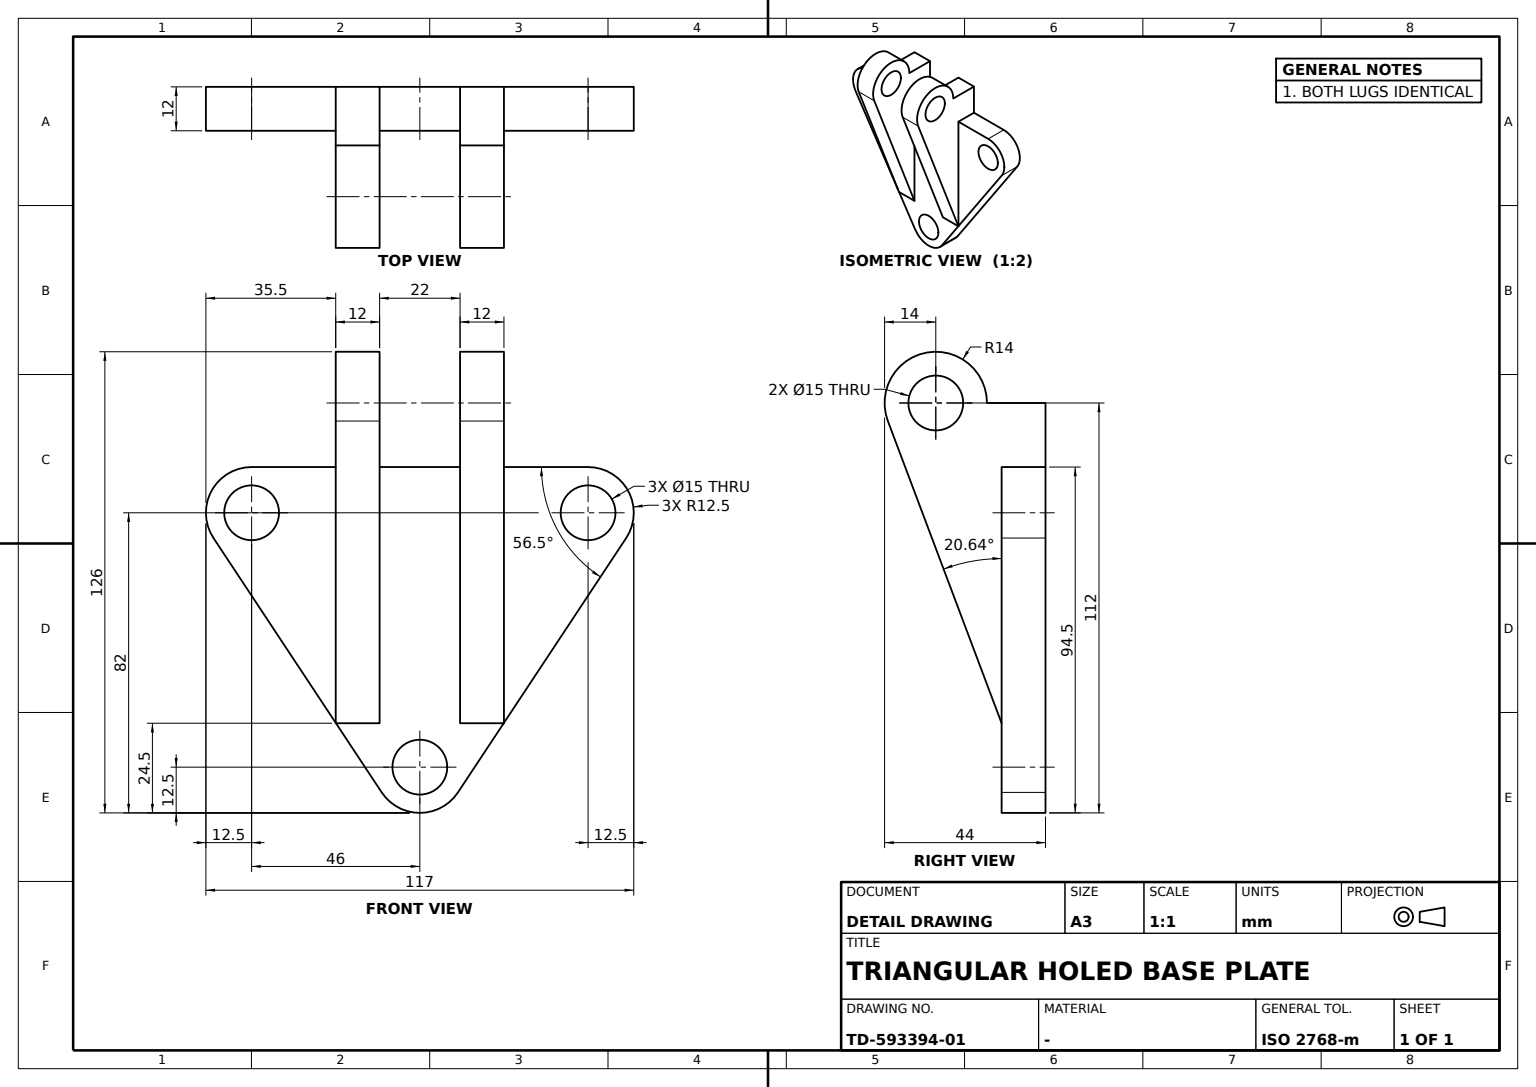
CATIA V5 part; units mm, degrees
sketch "Sketch1" plane through (0, 0, 0) normal (1, 0, 0) x (0, 1, 0)
  arc A0 (-46, 12.5) -> (-56.4236, -6.8991) centre (-46, 0) ccw
  point P0 (-46, 0)
  circle A1 centre (-46, 0) radius 7.5
  point P1 (46, 0)
  circle A2 centre (46, 0) radius 7.5
  arc A3 (46, 12.5) -> (56.4236, -6.8991) centre (46, 0) cw
  circle A4 centre (0, -69.5) radius 7.5
  point P2 (0, -69.5)
  arc A5 (-10.4236, -76.3991) -> (10.4236, -76.3991) centre (0, -69.5) ccw
  line L0 (-56.4236, -6.8991) -> (-10.4236, -76.3991)
  line L1 (10.4236, -76.3991) -> (56.4236, -6.8991)
  line L2 (-46, 12.5) -> (46, 12.5)
  dimension "radius A1" = 7.5
  dimension "radius A0" = 12.5
  dimension "distance P0 P1" = 92
  dimension "distance L2 P2" = 82
  constraint coincidence P0 x-axis
  constraint coincidence P2 y-axis
  constraint symmetry A1 A2 y-axis
  constraint symmetry A0 A3 y-axis
  constraint equal size A1 A4
  constraint equal size A0 A5
  constraint tangency L0 A0
  constraint tangency L0 A5
  constraint tangency L1 A5
  constraint tangency L1 A3
  constraint tangency L2 A0
  constraint tangency L2 A3
extrude "Pad1" add sketch "Sketch1" along normal blind 12
sketch "Sketch2" plane through (0, 0, 0) normal (0, 1, 0) x (-1, 0, 0)
  arc A0 (-16, 30) -> (-43.1013, 25.0649) centre (-30, 30) ccw
  point P0 (-30, 30)
  circle A1 centre (-30, 30) radius 7.5
  point P1 (-12, 12.5)
  line L0 (-12, 12.5) -> (-12, -57.5)
  line L1 (-12, -76.3991) -> (-12, -6.8991) construction
  line L2 (-43.1013, 25.0649) -> (-12, -57.5)
  line L3 (0, -6.8991) -> (0, 12.5) construction
  point P2 (-12, 12.5)
  line L4 (-16, 30) -> (0, 30)
  point P3 (0, 30)
  line L5 (0, 30) -> (0, 12.5)
  point P4 (-12, 12.5)
  line L6 (-12, 12.5) -> (0, 12.5)
  point P5 (0, -82)
  dimension "radius A1" = 7.5
  dimension "radius A0" = 14
  dimension "length L0" = 70
  dimension "distance L3 P0" = 30
  dimension "length L4" = 16
  dimension "distance P5 L4" = 112
  constraint vertical L0 y-axis
  constraint vertical L5 y-axis
  constraint coincidence L0 L1
  constraint coincidence P1 P2
  constraint coincidence P3 y-axis
  constraint coincidence P4 P1
  constraint tangency L2 A0
  constraint horizontal L4 x-axis
  constraint horizontal L6 x-axis
extrude "Pad2" add sketch "Sketch2" along normal blind 12 from surface at 11
mirror "Mirror1" about plane through (0, 0, 0) normal (0, 1, 0)
properties part number "Triangular Mounting Bracket with Double Fork Supports"
